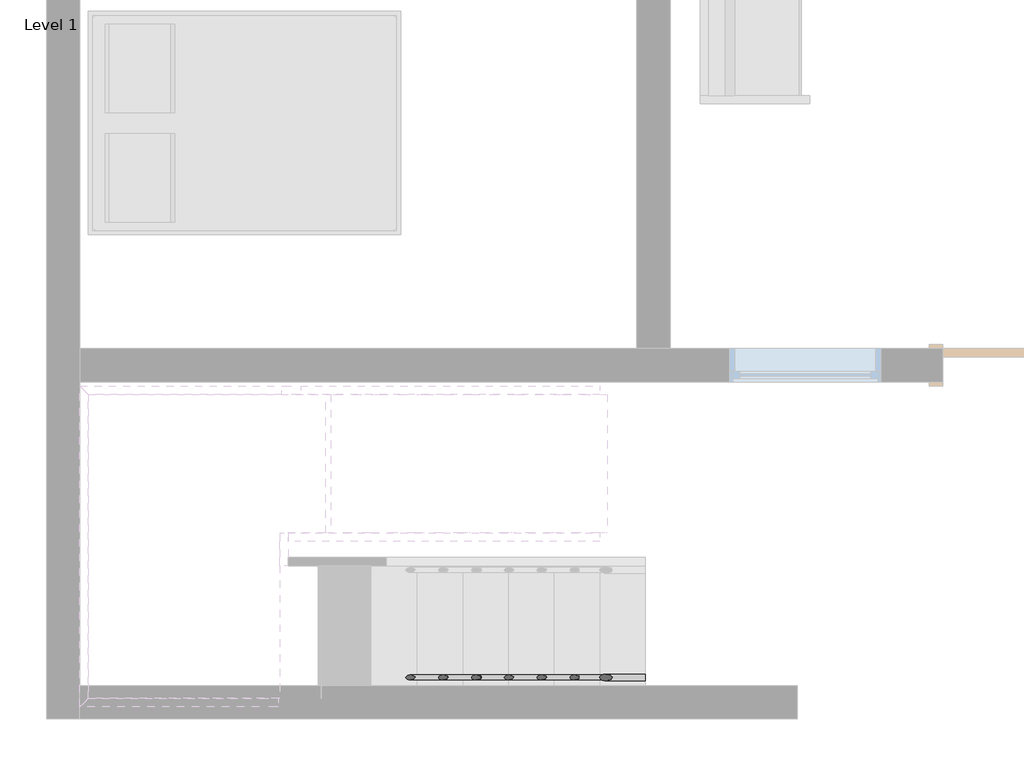
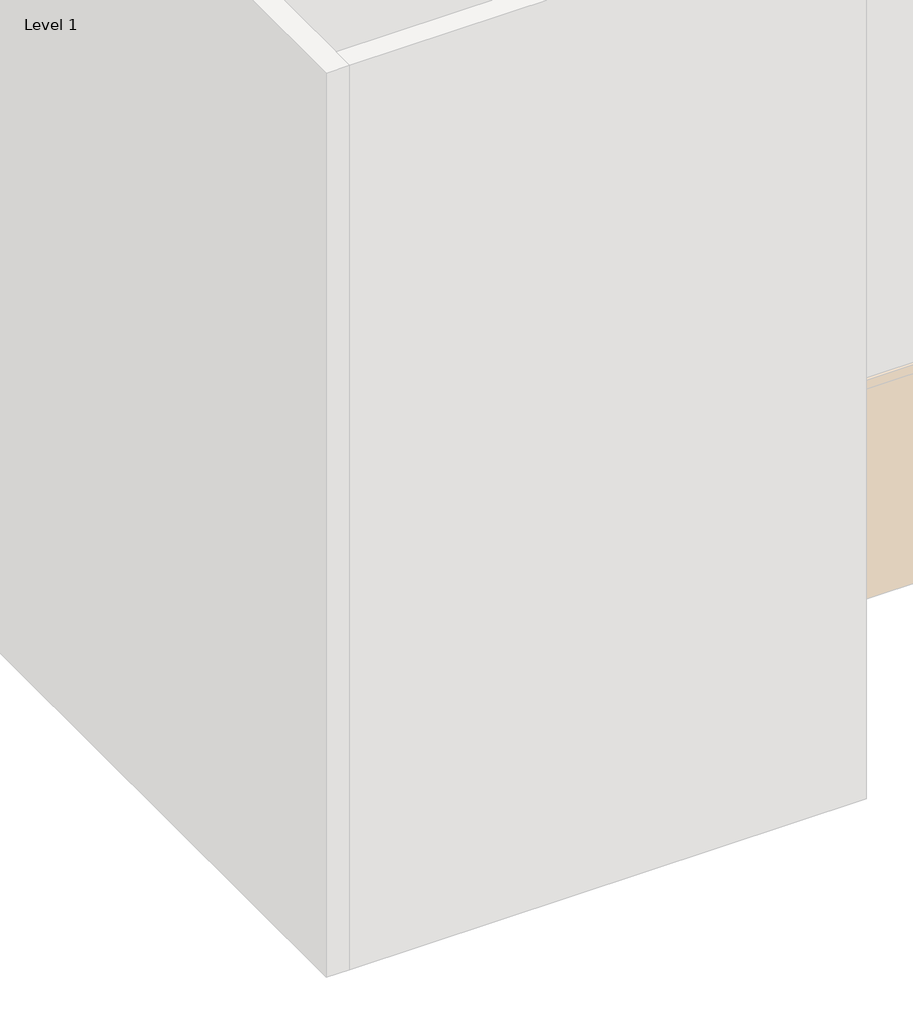
# One storey, part 3 of 4: 1 railing.
"""IFC4 building model written with IfcOpenShell, lengths in millimetres."""

from ifc_helpers import new_model, si_unit, point, frame, frame_2d, origin, place, context, project, spatial, circle_curve, ellipse_curve, trimmed, segment, composite_curve, outline, extrude, element, save
from ifc_brep_helpers import plane_surface, cylinder_surface, advanced_brep

model = new_model("IFC4")

# Units and contexts
model_context = context("Model", 3, world=origin())
ifc_project = project(units=[si_unit("LENGTHUNIT", "METRE", prefix="MILLI")], contexts=[model_context])

# Site, building, storey
site = spatial("IfcSite", under=ifc_project)
building = spatial("IfcBuilding", under=site)
storey = spatial("IfcBuildingStorey", under=building, Name="Level 1", Elevation=0.0)

# Railing
placement = place(None, origin())
element("IfcRailing", 1, ObjectType="900mm Pipe", at=placement, inside=storey, context=model_context, shape_type="SolidModel", body=[
    advanced_brep(
    [(-7153.6870075, 1559.2865734, 1050.2491997), (-7153.6870075, 1519.2865734, 1050.2491997), (-9359.4804605, 1559.2865734, 2445.2173913), (-9359.4804605, 1519.2865734, 2445.2173913), (-10462.6870075, 1559.2865734, 2445.2173913), (-10502.6870075, 1519.2865734, 2445.2173913), (-10462.6870075, 3300.4865734, 2445.2173913), (-10502.6870075, 3340.4865734, 2445.2173913), (-7428.6870075, 3300.4865734, 2445.2173913), (-7428.6870075, 3340.4865734, 2445.2173913)],
    [
        (0, 1, ellipse_curve(frame((-7153.6870075, 1539.2865734, 1050.2491997), z_axis=(1.0, 0.0, 0.0), x_axis=(0.0, 0.0, -1.0)), 23.6638438, 20.0)),
        (1, 0, ellipse_curve(frame((-7153.6870075, 1539.2865734, 1050.2491997), z_axis=(1.0, 0.0, 0.0), x_axis=(0.0, 0.0, -1.0)), 23.6638438, 20.0)),
        (0, 2),
        (2, 3, ellipse_curve(frame((-9359.4804605, 1539.2865734, 2445.2173913), z_axis=(0.9605132043335072, 0.0, -0.27823440531497556), x_axis=(-0.2782344053149751, 0.0, -0.9605132043335075)), 20.822202, 20.0)),
        (3, 1),
        (3, 2, ellipse_curve(frame((-9359.4804605, 1539.2865734, 2445.2173913), z_axis=(0.9605132043335072, 0.0, -0.27823440531497556), x_axis=(-0.2782344053149751, 0.0, -0.9605132043335075)), 20.822202, 20.0)),
        (2, 4),
        (4, 5, ellipse_curve(frame((-10482.6870075, 1539.2865734, 2445.2173913), z_axis=(0.7071067811865449, -0.70710678118655, 0.0), x_axis=(0.7071067811865501, 0.7071067811865448, 0.0)), 28.2842712, 20.0)),
        (5, 3),
        (5, 4, ellipse_curve(frame((-10482.6870075, 1539.2865734, 2445.2173913), z_axis=(0.7071067811865449, -0.70710678118655, 0.0), x_axis=(0.7071067811865501, 0.7071067811865448, 0.0)), 28.2842712, 20.0)),
        (4, 6),
        (6, 7, ellipse_curve(frame((-10482.6870075, 3320.4865734, 2445.2173913), z_axis=(-0.70710678118655, -0.7071067811865451, 0.0), x_axis=(0.7071067811865451, -0.7071067811865498, 0.0)), 28.2842712, 20.0)),
        (7, 5),
        (7, 6, ellipse_curve(frame((-10482.6870075, 3320.4865734, 2445.2173913), z_axis=(-0.70710678118655, -0.7071067811865451, 0.0), x_axis=(0.7071067811865451, -0.7071067811865498, 0.0)), 28.2842712, 20.0)),
        (8, 9, circle_curve(frame((-7428.6870075, 3320.4865734, 2445.2173913), z_axis=(1.0, 0.0, 0.0), x_axis=(0.0, 1.0, 0.0)), 20.0)),
        (9, 8, circle_curve(frame((-7428.6870075, 3320.4865734, 2445.2173913), z_axis=(1.0, 0.0, 0.0), x_axis=(0.0, 1.0, 0.0)), 20.0)),
        (6, 8),
        (9, 7),
    ],
    [
        plane_surface(frame((-7153.6870075, 1539.2865734, 1073.9130435), z_axis=(1.0, 0.0, 0.0), x_axis=(0.0, -1.0, 0.0))),
        cylinder_surface(frame((-7164.3769203, 1539.2865734, 1057.0096189), z_axis=(0.8451712313980437, 0.0, -0.5344956404098302), x_axis=(0.0, -1.0, 0.0)), 20.0),
        cylinder_surface(frame((-9353.6870075, 1539.2865734, 2445.2173913), z_axis=(1.0, 0.0, 0.0), x_axis=(0.0, -1.0, 0.0)), 20.0),
        cylinder_surface(frame((-10482.6870075, 1539.2865734, 2445.2173913), z_axis=(0.0, -1.0, 0.0), x_axis=(-1.0, 0.0, 0.0)), 20.0),
        plane_surface(frame((-7428.6870075, 3320.4865734, 2465.2173913), z_axis=(1.0, 0.0, 0.0), x_axis=(0.0, 1.0, 0.0))),
        cylinder_surface(frame((-10482.6870075, 3320.4865734, 2445.2173913), z_axis=(-1.0, 0.0, 0.0), x_axis=(0.0, 1.0, 0.0)), 20.0),
    ],
    [
        (0, [[1, 2]]),
        (1, [[-1, 3, 4, 5]]),
        (1, [[-2, -5, 6, -3]]),
        (2, [[-4, 7, 8, 9]]),
        (2, [[-6, -9, 10, -7]]),
        (3, [[-8, 11, 12, 13]]),
        (3, [[-10, -13, 14, -11]]),
        (4, [[15, 16]]),
        (5, [[-12, 17, -16, 18]]),
        (5, [[-14, -18, -15, -17]]),
    ],
),
    advanced_brep(
    [(-7153.6870075, 1554.2865734, 931.1651606), (-7153.6870075, 1524.2865734, 931.1651606), (-9358.0320973, 1554.2865734, 2325.2173913), (-9358.0320973, 1524.2865734, 2325.2173913), (-10467.6870075, 1554.2865734, 2325.2173913), (-10497.6870075, 1524.2865734, 2325.2173913), (-10467.6870075, 3305.4865734, 2325.2173913), (-10497.6870075, 3335.4865734, 2325.2173913), (-7428.6870075, 3305.4865734, 2325.2173913), (-7428.6870075, 3335.4865734, 2325.2173913)],
    [
        (0, 1, ellipse_curve(frame((-7153.6870075, 1539.2865734, 931.1651606), z_axis=(1.0, 0.0, 0.0), x_axis=(0.0, 0.0, -1.0)), 17.7478828, 15.0)),
        (1, 0, ellipse_curve(frame((-7153.6870075, 1539.2865734, 931.1651606), z_axis=(1.0, 0.0, 0.0), x_axis=(0.0, 0.0, -1.0)), 17.7478828, 15.0)),
        (0, 2),
        (2, 3, ellipse_curve(frame((-9358.0320973, 1539.2865734, 2325.2173913), z_axis=(0.9605132043335072, 0.0, -0.27823440531497556), x_axis=(-0.2782344053149751, 0.0, -0.9605132043335075)), 15.6166515, 15.0)),
        (3, 1),
        (3, 2, ellipse_curve(frame((-9358.0320973, 1539.2865734, 2325.2173913), z_axis=(0.9605132043335072, 0.0, -0.27823440531497556), x_axis=(-0.2782344053149751, 0.0, -0.9605132043335075)), 15.6166515, 15.0)),
        (2, 4),
        (4, 5, ellipse_curve(frame((-10482.6870075, 1539.2865734, 2325.2173913), z_axis=(0.7071067811865449, -0.70710678118655, 0.0), x_axis=(0.7071067811865501, 0.7071067811865448, 0.0)), 21.2132034, 15.0)),
        (5, 3),
        (5, 4, ellipse_curve(frame((-10482.6870075, 1539.2865734, 2325.2173913), z_axis=(0.7071067811865449, -0.70710678118655, 0.0), x_axis=(0.7071067811865501, 0.7071067811865448, 0.0)), 21.2132034, 15.0)),
        (4, 6),
        (6, 7, ellipse_curve(frame((-10482.6870075, 3320.4865734, 2325.2173913), z_axis=(-0.70710678118655, -0.7071067811865451, 0.0), x_axis=(0.7071067811865451, -0.7071067811865498, 0.0)), 21.2132034, 15.0)),
        (7, 5),
        (7, 6, ellipse_curve(frame((-10482.6870075, 3320.4865734, 2325.2173913), z_axis=(-0.70710678118655, -0.7071067811865451, 0.0), x_axis=(0.7071067811865451, -0.7071067811865498, 0.0)), 21.2132034, 15.0)),
        (8, 9, circle_curve(frame((-7428.6870075, 3320.4865734, 2325.2173913), z_axis=(1.0, 0.0, 0.0), x_axis=(0.0, 1.0, 0.0)), 15.0)),
        (9, 8, circle_curve(frame((-7428.6870075, 3320.4865734, 2325.2173913), z_axis=(1.0, 0.0, 0.0), x_axis=(0.0, 1.0, 0.0)), 15.0)),
        (6, 8),
        (9, 7),
    ],
    [
        plane_surface(frame((-7153.6870075, 1539.2865734, 948.9130435), z_axis=(1.0, 0.0, 0.0), x_axis=(0.0, -1.0, 0.0))),
        cylinder_surface(frame((-7161.7044421, 1539.2865734, 936.235475), z_axis=(0.8451712313980437, 0.0, -0.5344956404098302), x_axis=(0.0, -1.0, 0.0)), 15.0),
        cylinder_surface(frame((-9353.6870075, 1539.2865734, 2325.2173913), z_axis=(1.0, 0.0, 0.0), x_axis=(0.0, -1.0, 0.0)), 15.0),
        cylinder_surface(frame((-10482.6870075, 1539.2865734, 2325.2173913), z_axis=(0.0, -1.0, 0.0), x_axis=(-1.0, 0.0, 0.0)), 15.0),
        plane_surface(frame((-7428.6870075, 3320.4865734, 2340.2173913), z_axis=(1.0, 0.0, 0.0), x_axis=(0.0, 1.0, 0.0))),
        cylinder_surface(frame((-10482.6870075, 3320.4865734, 2325.2173913), z_axis=(-1.0, 0.0, 0.0), x_axis=(0.0, 1.0, 0.0)), 15.0),
    ],
    [
        (0, [[1, 2]]),
        (1, [[-1, 3, 4, 5]]),
        (1, [[-2, -5, 6, -3]]),
        (2, [[-4, 7, 8, 9]]),
        (2, [[-6, -9, 10, -7]]),
        (3, [[-8, 11, 12, 13]]),
        (3, [[-10, -13, 14, -11]]),
        (4, [[15, 16]]),
        (5, [[-12, 17, -16, 18]]),
        (5, [[-14, -18, -15, -17]]),
    ],
),
    advanced_brep(
    [(-7153.6870075, 1554.2865734, 806.1651606), (-7153.6870075, 1524.2865734, 806.1651606), (-9358.0320973, 1554.2865734, 2200.2173913), (-9358.0320973, 1524.2865734, 2200.2173913), (-10467.6870075, 1554.2865734, 2200.2173913), (-10497.6870075, 1524.2865734, 2200.2173913), (-10467.6870075, 3305.4865734, 2200.2173913), (-10497.6870075, 3335.4865734, 2200.2173913), (-7428.6870075, 3305.4865734, 2200.2173913), (-7428.6870075, 3335.4865734, 2200.2173913)],
    [
        (0, 1, ellipse_curve(frame((-7153.6870075, 1539.2865734, 806.1651606), z_axis=(1.0, 0.0, 0.0), x_axis=(0.0, 0.0, -1.0)), 17.7478828, 15.0)),
        (1, 0, ellipse_curve(frame((-7153.6870075, 1539.2865734, 806.1651606), z_axis=(1.0, 0.0, 0.0), x_axis=(0.0, 0.0, -1.0)), 17.7478828, 15.0)),
        (0, 2),
        (2, 3, ellipse_curve(frame((-9358.0320973, 1539.2865734, 2200.2173913), z_axis=(0.9605132043335072, 0.0, -0.27823440531497556), x_axis=(-0.2782344053149751, 0.0, -0.9605132043335075)), 15.6166515, 15.0)),
        (3, 1),
        (3, 2, ellipse_curve(frame((-9358.0320973, 1539.2865734, 2200.2173913), z_axis=(0.9605132043335072, 0.0, -0.27823440531497556), x_axis=(-0.2782344053149751, 0.0, -0.9605132043335075)), 15.6166515, 15.0)),
        (2, 4),
        (4, 5, ellipse_curve(frame((-10482.6870075, 1539.2865734, 2200.2173913), z_axis=(0.7071067811865449, -0.70710678118655, 0.0), x_axis=(0.7071067811865501, 0.7071067811865448, 0.0)), 21.2132034, 15.0)),
        (5, 3),
        (5, 4, ellipse_curve(frame((-10482.6870075, 1539.2865734, 2200.2173913), z_axis=(0.7071067811865449, -0.70710678118655, 0.0), x_axis=(0.7071067811865501, 0.7071067811865448, 0.0)), 21.2132034, 15.0)),
        (4, 6),
        (6, 7, ellipse_curve(frame((-10482.6870075, 3320.4865734, 2200.2173913), z_axis=(-0.70710678118655, -0.7071067811865451, 0.0), x_axis=(0.7071067811865451, -0.7071067811865498, 0.0)), 21.2132034, 15.0)),
        (7, 5),
        (7, 6, ellipse_curve(frame((-10482.6870075, 3320.4865734, 2200.2173913), z_axis=(-0.70710678118655, -0.7071067811865451, 0.0), x_axis=(0.7071067811865451, -0.7071067811865498, 0.0)), 21.2132034, 15.0)),
        (8, 9, circle_curve(frame((-7428.6870075, 3320.4865734, 2200.2173913), z_axis=(1.0, 0.0, 0.0), x_axis=(0.0, 1.0, 0.0)), 15.0)),
        (9, 8, circle_curve(frame((-7428.6870075, 3320.4865734, 2200.2173913), z_axis=(1.0, 0.0, 0.0), x_axis=(0.0, 1.0, 0.0)), 15.0)),
        (6, 8),
        (9, 7),
    ],
    [
        plane_surface(frame((-7153.6870075, 1539.2865734, 823.9130435), z_axis=(1.0, 0.0, 0.0), x_axis=(0.0, -1.0, 0.0))),
        cylinder_surface(frame((-7161.7044421, 1539.2865734, 811.235475), z_axis=(0.8451712313980437, 0.0, -0.5344956404098302), x_axis=(0.0, -1.0, 0.0)), 15.0),
        cylinder_surface(frame((-9353.6870075, 1539.2865734, 2200.2173913), z_axis=(1.0, 0.0, 0.0), x_axis=(0.0, -1.0, 0.0)), 15.0),
        cylinder_surface(frame((-10482.6870075, 1539.2865734, 2200.2173913), z_axis=(0.0, -1.0, 0.0), x_axis=(-1.0, 0.0, 0.0)), 15.0),
        plane_surface(frame((-7428.6870075, 3320.4865734, 2215.2173913), z_axis=(1.0, 0.0, 0.0), x_axis=(0.0, 1.0, 0.0))),
        cylinder_surface(frame((-10482.6870075, 3320.4865734, 2200.2173913), z_axis=(-1.0, 0.0, 0.0), x_axis=(0.0, 1.0, 0.0)), 15.0),
    ],
    [
        (0, [[1, 2]]),
        (1, [[-1, 3, 4, 5]]),
        (1, [[-2, -5, 6, -3]]),
        (2, [[-4, 7, 8, 9]]),
        (2, [[-6, -9, 10, -7]]),
        (3, [[-8, 11, 12, 13]]),
        (3, [[-10, -13, 14, -11]]),
        (4, [[15, 16]]),
        (5, [[-12, 17, -16, 18]]),
        (5, [[-14, -18, -15, -17]]),
    ],
),
    advanced_brep(
    [(-7153.6870075, 1554.2865734, 681.1651606), (-7153.6870075, 1524.2865734, 681.1651606), (-9358.0320973, 1554.2865734, 2075.2173913), (-9358.0320973, 1524.2865734, 2075.2173913), (-10467.6870075, 1554.2865734, 2075.2173913), (-10497.6870075, 1524.2865734, 2075.2173913), (-10467.6870075, 3305.4865734, 2075.2173913), (-10497.6870075, 3335.4865734, 2075.2173913), (-7428.6870075, 3305.4865734, 2075.2173913), (-7428.6870075, 3335.4865734, 2075.2173913)],
    [
        (0, 1, ellipse_curve(frame((-7153.6870075, 1539.2865734, 681.1651606), z_axis=(1.0, 0.0, 0.0), x_axis=(0.0, 0.0, -1.0)), 17.7478828, 15.0)),
        (1, 0, ellipse_curve(frame((-7153.6870075, 1539.2865734, 681.1651606), z_axis=(1.0, 0.0, 0.0), x_axis=(0.0, 0.0, -1.0)), 17.7478828, 15.0)),
        (0, 2),
        (2, 3, ellipse_curve(frame((-9358.0320973, 1539.2865734, 2075.2173913), z_axis=(0.9605132043335072, 0.0, -0.27823440531497556), x_axis=(-0.2782344053149751, 0.0, -0.9605132043335075)), 15.6166515, 15.0)),
        (3, 1),
        (3, 2, ellipse_curve(frame((-9358.0320973, 1539.2865734, 2075.2173913), z_axis=(0.9605132043335072, 0.0, -0.27823440531497556), x_axis=(-0.2782344053149751, 0.0, -0.9605132043335075)), 15.6166515, 15.0)),
        (2, 4),
        (4, 5, ellipse_curve(frame((-10482.6870075, 1539.2865734, 2075.2173913), z_axis=(0.7071067811865449, -0.70710678118655, 0.0), x_axis=(0.7071067811865501, 0.7071067811865448, 0.0)), 21.2132034, 15.0)),
        (5, 3),
        (5, 4, ellipse_curve(frame((-10482.6870075, 1539.2865734, 2075.2173913), z_axis=(0.7071067811865449, -0.70710678118655, 0.0), x_axis=(0.7071067811865501, 0.7071067811865448, 0.0)), 21.2132034, 15.0)),
        (4, 6),
        (6, 7, ellipse_curve(frame((-10482.6870075, 3320.4865734, 2075.2173913), z_axis=(-0.70710678118655, -0.7071067811865451, 0.0), x_axis=(0.7071067811865451, -0.7071067811865498, 0.0)), 21.2132034, 15.0)),
        (7, 5),
        (7, 6, ellipse_curve(frame((-10482.6870075, 3320.4865734, 2075.2173913), z_axis=(-0.70710678118655, -0.7071067811865451, 0.0), x_axis=(0.7071067811865451, -0.7071067811865498, 0.0)), 21.2132034, 15.0)),
        (8, 9, circle_curve(frame((-7428.6870075, 3320.4865734, 2075.2173913), z_axis=(1.0, 0.0, 0.0), x_axis=(0.0, 1.0, 0.0)), 15.0)),
        (9, 8, circle_curve(frame((-7428.6870075, 3320.4865734, 2075.2173913), z_axis=(1.0, 0.0, 0.0), x_axis=(0.0, 1.0, 0.0)), 15.0)),
        (6, 8),
        (9, 7),
    ],
    [
        plane_surface(frame((-7153.6870075, 1539.2865734, 698.9130435), z_axis=(1.0, 0.0, 0.0), x_axis=(0.0, -1.0, 0.0))),
        cylinder_surface(frame((-7161.7044421, 1539.2865734, 686.235475), z_axis=(0.8451712313980437, 0.0, -0.5344956404098302), x_axis=(0.0, -1.0, 0.0)), 15.0),
        cylinder_surface(frame((-9353.6870075, 1539.2865734, 2075.2173913), z_axis=(1.0, 0.0, 0.0), x_axis=(0.0, -1.0, 0.0)), 15.0),
        cylinder_surface(frame((-10482.6870075, 1539.2865734, 2075.2173913), z_axis=(0.0, -1.0, 0.0), x_axis=(-1.0, 0.0, 0.0)), 15.0),
        plane_surface(frame((-7428.6870075, 3320.4865734, 2090.2173913), z_axis=(1.0, 0.0, 0.0), x_axis=(0.0, 1.0, 0.0))),
        cylinder_surface(frame((-10482.6870075, 3320.4865734, 2075.2173913), z_axis=(-1.0, 0.0, 0.0), x_axis=(0.0, 1.0, 0.0)), 15.0),
    ],
    [
        (0, [[1, 2]]),
        (1, [[-1, 3, 4, 5]]),
        (1, [[-2, -5, 6, -3]]),
        (2, [[-4, 7, 8, 9]]),
        (2, [[-6, -9, 10, -7]]),
        (3, [[-8, 11, 12, 13]]),
        (3, [[-10, -13, 14, -11]]),
        (4, [[15, 16]]),
        (5, [[-12, 17, -16, 18]]),
        (5, [[-14, -18, -15, -17]]),
    ],
),
    advanced_brep(
    [(-7153.6870075, 1554.2865734, 556.1651606), (-7153.6870075, 1524.2865734, 556.1651606), (-9358.0320973, 1554.2865734, 1950.2173913), (-9358.0320973, 1524.2865734, 1950.2173913), (-10467.6870075, 1554.2865734, 1950.2173913), (-10497.6870075, 1524.2865734, 1950.2173913), (-10467.6870075, 3305.4865734, 1950.2173913), (-10497.6870075, 3335.4865734, 1950.2173913), (-7428.6870075, 3305.4865734, 1950.2173913), (-7428.6870075, 3335.4865734, 1950.2173913)],
    [
        (0, 1, ellipse_curve(frame((-7153.6870075, 1539.2865734, 556.1651606), z_axis=(1.0, 0.0, 0.0), x_axis=(0.0, 0.0, -1.0)), 17.7478828, 15.0)),
        (1, 0, ellipse_curve(frame((-7153.6870075, 1539.2865734, 556.1651606), z_axis=(1.0, 0.0, 0.0), x_axis=(0.0, 0.0, -1.0)), 17.7478828, 15.0)),
        (0, 2),
        (2, 3, ellipse_curve(frame((-9358.0320973, 1539.2865734, 1950.2173913), z_axis=(0.9605132043335072, 0.0, -0.27823440531497556), x_axis=(-0.2782344053149751, 0.0, -0.9605132043335075)), 15.6166515, 15.0)),
        (3, 1),
        (3, 2, ellipse_curve(frame((-9358.0320973, 1539.2865734, 1950.2173913), z_axis=(0.9605132043335072, 0.0, -0.27823440531497556), x_axis=(-0.2782344053149751, 0.0, -0.9605132043335075)), 15.6166515, 15.0)),
        (2, 4),
        (4, 5, ellipse_curve(frame((-10482.6870075, 1539.2865734, 1950.2173913), z_axis=(0.7071067811865449, -0.70710678118655, 0.0), x_axis=(0.7071067811865501, 0.7071067811865448, 0.0)), 21.2132034, 15.0)),
        (5, 3),
        (5, 4, ellipse_curve(frame((-10482.6870075, 1539.2865734, 1950.2173913), z_axis=(0.7071067811865449, -0.70710678118655, 0.0), x_axis=(0.7071067811865501, 0.7071067811865448, 0.0)), 21.2132034, 15.0)),
        (4, 6),
        (6, 7, ellipse_curve(frame((-10482.6870075, 3320.4865734, 1950.2173913), z_axis=(-0.70710678118655, -0.7071067811865451, 0.0), x_axis=(0.7071067811865451, -0.7071067811865498, 0.0)), 21.2132034, 15.0)),
        (7, 5),
        (7, 6, ellipse_curve(frame((-10482.6870075, 3320.4865734, 1950.2173913), z_axis=(-0.70710678118655, -0.7071067811865451, 0.0), x_axis=(0.7071067811865451, -0.7071067811865498, 0.0)), 21.2132034, 15.0)),
        (8, 9, circle_curve(frame((-7428.6870075, 3320.4865734, 1950.2173913), z_axis=(1.0, 0.0, 0.0), x_axis=(0.0, 1.0, 0.0)), 15.0)),
        (9, 8, circle_curve(frame((-7428.6870075, 3320.4865734, 1950.2173913), z_axis=(1.0, 0.0, 0.0), x_axis=(0.0, 1.0, 0.0)), 15.0)),
        (6, 8),
        (9, 7),
    ],
    [
        plane_surface(frame((-7153.6870075, 1539.2865734, 573.9130435), z_axis=(1.0, 0.0, 0.0), x_axis=(0.0, -1.0, 0.0))),
        cylinder_surface(frame((-7161.7044421, 1539.2865734, 561.235475), z_axis=(0.8451712313980437, 0.0, -0.5344956404098302), x_axis=(0.0, -1.0, 0.0)), 15.0),
        cylinder_surface(frame((-9353.6870075, 1539.2865734, 1950.2173913), z_axis=(1.0, 0.0, 0.0), x_axis=(0.0, -1.0, 0.0)), 15.0),
        cylinder_surface(frame((-10482.6870075, 1539.2865734, 1950.2173913), z_axis=(0.0, -1.0, 0.0), x_axis=(-1.0, 0.0, 0.0)), 15.0),
        plane_surface(frame((-7428.6870075, 3320.4865734, 1965.2173913), z_axis=(1.0, 0.0, 0.0), x_axis=(0.0, 1.0, 0.0))),
        cylinder_surface(frame((-10482.6870075, 3320.4865734, 1950.2173913), z_axis=(-1.0, 0.0, 0.0), x_axis=(0.0, 1.0, 0.0)), 15.0),
    ],
    [
        (0, [[1, 2]]),
        (1, [[-1, 3, 4, 5]]),
        (1, [[-2, -5, 6, -3]]),
        (2, [[-4, 7, 8, 9]]),
        (2, [[-6, -9, 10, -7]]),
        (3, [[-8, 11, 12, 13]]),
        (3, [[-10, -13, 14, -11]]),
        (4, [[15, 16]]),
        (5, [[-12, 17, -16, 18]]),
        (5, [[-14, -18, -15, -17]]),
    ],
),
    advanced_brep(
    [(-7153.6870075, 1554.2865734, 431.1651606), (-7153.6870075, 1524.2865734, 431.1651606), (-9358.0320973, 1554.2865734, 1825.2173913), (-9358.0320973, 1524.2865734, 1825.2173913), (-10467.6870075, 1554.2865734, 1825.2173913), (-10497.6870075, 1524.2865734, 1825.2173913), (-10467.6870075, 3305.4865734, 1825.2173913), (-10497.6870075, 3335.4865734, 1825.2173913), (-7428.6870075, 3305.4865734, 1825.2173913), (-7428.6870075, 3335.4865734, 1825.2173913)],
    [
        (0, 1, ellipse_curve(frame((-7153.6870075, 1539.2865734, 431.1651606), z_axis=(1.0, 0.0, 0.0), x_axis=(0.0, 0.0, -1.0)), 17.7478828, 15.0)),
        (1, 0, ellipse_curve(frame((-7153.6870075, 1539.2865734, 431.1651606), z_axis=(1.0, 0.0, 0.0), x_axis=(0.0, 0.0, -1.0)), 17.7478828, 15.0)),
        (0, 2),
        (2, 3, ellipse_curve(frame((-9358.0320973, 1539.2865734, 1825.2173913), z_axis=(0.9605132043335072, 0.0, -0.27823440531497556), x_axis=(-0.2782344053149751, 0.0, -0.9605132043335075)), 15.6166515, 15.0)),
        (3, 1),
        (3, 2, ellipse_curve(frame((-9358.0320973, 1539.2865734, 1825.2173913), z_axis=(0.9605132043335072, 0.0, -0.27823440531497556), x_axis=(-0.2782344053149751, 0.0, -0.9605132043335075)), 15.6166515, 15.0)),
        (2, 4),
        (4, 5, ellipse_curve(frame((-10482.6870075, 1539.2865734, 1825.2173913), z_axis=(0.7071067811865449, -0.70710678118655, 0.0), x_axis=(0.7071067811865501, 0.7071067811865448, 0.0)), 21.2132034, 15.0)),
        (5, 3),
        (5, 4, ellipse_curve(frame((-10482.6870075, 1539.2865734, 1825.2173913), z_axis=(0.7071067811865449, -0.70710678118655, 0.0), x_axis=(0.7071067811865501, 0.7071067811865448, 0.0)), 21.2132034, 15.0)),
        (4, 6),
        (6, 7, ellipse_curve(frame((-10482.6870075, 3320.4865734, 1825.2173913), z_axis=(-0.70710678118655, -0.7071067811865451, 0.0), x_axis=(0.7071067811865451, -0.7071067811865498, 0.0)), 21.2132034, 15.0)),
        (7, 5),
        (7, 6, ellipse_curve(frame((-10482.6870075, 3320.4865734, 1825.2173913), z_axis=(-0.70710678118655, -0.7071067811865451, 0.0), x_axis=(0.7071067811865451, -0.7071067811865498, 0.0)), 21.2132034, 15.0)),
        (8, 9, circle_curve(frame((-7428.6870075, 3320.4865734, 1825.2173913), z_axis=(1.0, 0.0, 0.0), x_axis=(0.0, 1.0, 0.0)), 15.0)),
        (9, 8, circle_curve(frame((-7428.6870075, 3320.4865734, 1825.2173913), z_axis=(1.0, 0.0, 0.0), x_axis=(0.0, 1.0, 0.0)), 15.0)),
        (6, 8),
        (9, 7),
    ],
    [
        plane_surface(frame((-7153.6870075, 1539.2865734, 448.9130435), z_axis=(1.0, 0.0, 0.0), x_axis=(0.0, -1.0, 0.0))),
        cylinder_surface(frame((-7161.7044421, 1539.2865734, 436.235475), z_axis=(0.8451712313980437, 0.0, -0.5344956404098302), x_axis=(0.0, -1.0, 0.0)), 15.0),
        cylinder_surface(frame((-9353.6870075, 1539.2865734, 1825.2173913), z_axis=(1.0, 0.0, 0.0), x_axis=(0.0, -1.0, 0.0)), 15.0),
        cylinder_surface(frame((-10482.6870075, 1539.2865734, 1825.2173913), z_axis=(0.0, -1.0, 0.0), x_axis=(-1.0, 0.0, 0.0)), 15.0),
        plane_surface(frame((-7428.6870075, 3320.4865734, 1840.2173913), z_axis=(1.0, 0.0, 0.0), x_axis=(0.0, 1.0, 0.0))),
        cylinder_surface(frame((-10482.6870075, 3320.4865734, 1825.2173913), z_axis=(-1.0, 0.0, 0.0), x_axis=(0.0, 1.0, 0.0)), 15.0),
    ],
    [
        (0, [[1, 2]]),
        (1, [[-1, 3, 4, 5]]),
        (1, [[-2, -5, 6, -3]]),
        (2, [[-4, 7, 8, 9]]),
        (2, [[-6, -9, 10, -7]]),
        (3, [[-8, 11, 12, 13]]),
        (3, [[-10, -13, 14, -11]]),
        (4, [[15, 16]]),
        (5, [[-12, 17, -16, 18]]),
        (5, [[-14, -18, -15, -17]]),
    ],
),
    advanced_brep(
    [(-7153.6870075, 1554.2865734, 306.1651606), (-7153.6870075, 1524.2865734, 306.1651606), (-9358.0320973, 1554.2865734, 1700.2173913), (-9358.0320973, 1524.2865734, 1700.2173913), (-10467.6870075, 1554.2865734, 1700.2173913), (-10497.6870075, 1524.2865734, 1700.2173913), (-10467.6870075, 3305.4865734, 1700.2173913), (-10497.6870075, 3335.4865734, 1700.2173913), (-7428.6870075, 3305.4865734, 1700.2173913), (-7428.6870075, 3335.4865734, 1700.2173913)],
    [
        (0, 1, ellipse_curve(frame((-7153.6870075, 1539.2865734, 306.1651606), z_axis=(1.0, 0.0, 0.0), x_axis=(0.0, 0.0, -1.0)), 17.7478828, 15.0)),
        (1, 0, ellipse_curve(frame((-7153.6870075, 1539.2865734, 306.1651606), z_axis=(1.0, 0.0, 0.0), x_axis=(0.0, 0.0, -1.0)), 17.7478828, 15.0)),
        (0, 2),
        (2, 3, ellipse_curve(frame((-9358.0320973, 1539.2865734, 1700.2173913), z_axis=(0.9605132043335072, 0.0, -0.27823440531497556), x_axis=(-0.2782344053149751, 0.0, -0.9605132043335075)), 15.6166515, 15.0)),
        (3, 1),
        (3, 2, ellipse_curve(frame((-9358.0320973, 1539.2865734, 1700.2173913), z_axis=(0.9605132043335072, 0.0, -0.27823440531497556), x_axis=(-0.2782344053149751, 0.0, -0.9605132043335075)), 15.6166515, 15.0)),
        (2, 4),
        (4, 5, ellipse_curve(frame((-10482.6870075, 1539.2865734, 1700.2173913), z_axis=(0.7071067811865449, -0.70710678118655, 0.0), x_axis=(0.7071067811865501, 0.7071067811865448, 0.0)), 21.2132034, 15.0)),
        (5, 3),
        (5, 4, ellipse_curve(frame((-10482.6870075, 1539.2865734, 1700.2173913), z_axis=(0.7071067811865449, -0.70710678118655, 0.0), x_axis=(0.7071067811865501, 0.7071067811865448, 0.0)), 21.2132034, 15.0)),
        (4, 6),
        (6, 7, ellipse_curve(frame((-10482.6870075, 3320.4865734, 1700.2173913), z_axis=(-0.70710678118655, -0.7071067811865451, 0.0), x_axis=(0.7071067811865451, -0.7071067811865498, 0.0)), 21.2132034, 15.0)),
        (7, 5),
        (7, 6, ellipse_curve(frame((-10482.6870075, 3320.4865734, 1700.2173913), z_axis=(-0.70710678118655, -0.7071067811865451, 0.0), x_axis=(0.7071067811865451, -0.7071067811865498, 0.0)), 21.2132034, 15.0)),
        (8, 9, circle_curve(frame((-7428.6870075, 3320.4865734, 1700.2173913), z_axis=(1.0, 0.0, 0.0), x_axis=(0.0, 1.0, 0.0)), 15.0)),
        (9, 8, circle_curve(frame((-7428.6870075, 3320.4865734, 1700.2173913), z_axis=(1.0, 0.0, 0.0), x_axis=(0.0, 1.0, 0.0)), 15.0)),
        (6, 8),
        (9, 7),
    ],
    [
        plane_surface(frame((-7153.6870075, 1539.2865734, 323.9130435), z_axis=(1.0, 0.0, 0.0), x_axis=(0.0, -1.0, 0.0))),
        cylinder_surface(frame((-7161.7044421, 1539.2865734, 311.235475), z_axis=(0.8451712313980437, 0.0, -0.5344956404098302), x_axis=(0.0, -1.0, 0.0)), 15.0),
        cylinder_surface(frame((-9353.6870075, 1539.2865734, 1700.2173913), z_axis=(1.0, 0.0, 0.0), x_axis=(0.0, -1.0, 0.0)), 15.0),
        cylinder_surface(frame((-10482.6870075, 1539.2865734, 1700.2173913), z_axis=(0.0, -1.0, 0.0), x_axis=(-1.0, 0.0, 0.0)), 15.0),
        plane_surface(frame((-7428.6870075, 3320.4865734, 1715.2173913), z_axis=(1.0, 0.0, 0.0), x_axis=(0.0, 1.0, 0.0))),
        cylinder_surface(frame((-10482.6870075, 3320.4865734, 1700.2173913), z_axis=(-1.0, 0.0, 0.0), x_axis=(0.0, 1.0, 0.0)), 15.0),
    ],
    [
        (0, [[1, 2]]),
        (1, [[-1, 3, 4, 5]]),
        (1, [[-2, -5, 6, -3]]),
        (2, [[-4, 7, 8, 9]]),
        (2, [[-6, -9, 10, -7]]),
        (3, [[-8, 11, 12, 13]]),
        (3, [[-10, -13, 14, -11]]),
        (4, [[15, 16]]),
        (5, [[-12, 17, -16, 18]]),
        (5, [[-14, -18, -15, -17]]),
    ],
),
    extrude(outline(composite_curve([segment(trimmed(circle_curve(frame_2d((-8078.6870075, 3320.4865734)), 12.5), [point((-8078.6870075, 3307.9865734))], [point((-8078.6870075, 3332.9865734))], False, "CARTESIAN"), True, "CONTINUOUS"), segment(trimmed(circle_curve(frame_2d((-8078.6870075, 3320.4865734)), 12.5), [point((-8078.6870075, 3332.9865734))], [point((-8078.6870075, 3307.9865734))], False, "CARTESIAN"), True, "CONTINUOUS")], self_intersect=False)), frame((0.0, 0.0, 1565.2173913), z_axis=(0.0, 0.0, 1.0), x_axis=(1.0, 0.0, 0.0)), (0.0, 0.0, 1.0), 860.0),
    extrude(outline(composite_curve([segment(trimmed(circle_curve(frame_2d((-9482.6870075, 3320.4865734)), 12.5), [point((-9482.6870075, 3307.9865734))], [point((-9482.6870075, 3332.9865734))], False, "CARTESIAN"), True, "CONTINUOUS"), segment(trimmed(circle_curve(frame_2d((-9482.6870075, 3320.4865734)), 12.5), [point((-9482.6870075, 3332.9865734))], [point((-9482.6870075, 3307.9865734))], False, "CARTESIAN"), True, "CONTINUOUS")], self_intersect=False)), frame((0.0, 0.0, 1565.2173913), z_axis=(0.0, 0.0, 1.0), x_axis=(1.0, 0.0, 0.0)), (0.0, 0.0, 1.0), 860.0),
    extrude(outline(composite_curve([segment(trimmed(circle_curve(frame_2d((-10482.6870075, 2539.2865734)), 12.5), [point((-10470.1870075, 2539.2865734))], [point((-10495.1870075, 2539.2865734))], False, "CARTESIAN"), True, "CONTINUOUS"), segment(trimmed(circle_curve(frame_2d((-10482.6870075, 2539.2865734)), 12.5), [point((-10495.1870075, 2539.2865734))], [point((-10470.1870075, 2539.2865734))], False, "CARTESIAN"), True, "CONTINUOUS")], self_intersect=False)), frame((0.0, 0.0, 1565.2173913), z_axis=(0.0, 0.0, 1.0), x_axis=(1.0, 0.0, 0.0)), (0.0, 0.0, 1.0), 860.0),
    extrude(outline(composite_curve([segment(trimmed(circle_curve(frame_2d((-10353.6870075, 1539.2865734)), 12.5), [point((-10353.6870075, 1551.7865734))], [point((-10353.6870075, 1526.7865734))], False, "CARTESIAN"), True, "CONTINUOUS"), segment(trimmed(circle_curve(frame_2d((-10353.6870075, 1539.2865734)), 12.5), [point((-10353.6870075, 1526.7865734))], [point((-10353.6870075, 1551.7865734))], False, "CARTESIAN"), True, "CONTINUOUS")], self_intersect=False)), frame((0.0, 0.0, 1565.2173913), z_axis=(0.0, 0.0, 1.0), x_axis=(1.0, 0.0, 0.0)), (0.0, 0.0, 1.0), 860.0),
    advanced_brep(
    [(-9153.6870075, 1526.7865734, 2291.4074903), (-9153.6870075, 1551.7865734, 2291.4074903), (-9153.6870075, 1551.7865734, 1391.3043478), (-9153.6870075, 1526.7865734, 1391.3043478)],
    [
        (0, 1, ellipse_curve(frame((-9153.6870075, 1539.2865734, 2291.4074903), z_axis=(-0.5344956404098302, 0.0, -0.8451712313980437), x_axis=(-0.8451712313980437, 0.0, 0.53449564040983)), 14.7899024, 12.5)),
        (1, 2),
        (2, 3, circle_curve(frame((-9153.6870075, 1539.2865734, 1391.3043478), z_axis=(0.0, 0.0, 1.0), x_axis=(0.0, 1.0, 0.0)), 12.5)),
        (3, 0),
        (3, 2, circle_curve(frame((-9153.6870075, 1539.2865734, 1391.3043478), z_axis=(0.0, 0.0, 1.0), x_axis=(0.0, 1.0, 0.0)), 12.5)),
        (1, 0, ellipse_curve(frame((-9153.6870075, 1539.2865734, 2291.4074903), z_axis=(-0.5344956404098302, 0.0, -0.8451712313980437), x_axis=(-0.8451712313980437, 0.0, 0.53449564040983)), 14.7899024, 12.5)),
    ],
    [
        cylinder_surface(frame((-9153.6870075, 1539.2865734, 1291.3043478), z_axis=(0.0, 0.0, 1.0), x_axis=(0.0, 1.0, 0.0)), 12.5),
        plane_surface(frame((-9178.6870075, 1564.2865734, 2307.217767), z_axis=(0.5344956404098302, 0.0, 0.8451712313980437), x_axis=(0.0, -1.0, 0.0))),
        plane_surface(frame((-9128.6870075, 1564.2865734, 1391.3043478), z_axis=(0.0, 0.0, -1.0), x_axis=(0.0, -1.0, 0.0))),
    ],
    [
        (0, [[1, 2, 3, 4]]),
        (0, [[5, -2, 6, -4]]),
        (1, [[-6, -1]]),
        (2, [[-5, -3]]),
    ],
),
    advanced_brep(
    [(-8153.6870075, 1526.7865734, 1658.9964231), (-8153.6870075, 1551.7865734, 1658.9964231), (-8153.6870075, 1551.7865734, 695.6521739), (-8153.6870075, 1526.7865734, 695.6521739)],
    [
        (0, 1, ellipse_curve(frame((-8153.6870075, 1539.2865734, 1658.9964231), z_axis=(-0.5344956404098302, 0.0, -0.8451712313980437), x_axis=(-0.8451712313980437, 0.0, 0.53449564040983)), 14.7899024, 12.5)),
        (1, 2),
        (2, 3, circle_curve(frame((-8153.6870075, 1539.2865734, 695.6521739), z_axis=(0.0, 0.0, 1.0), x_axis=(0.0, 1.0, 0.0)), 12.5)),
        (3, 0),
        (3, 2, circle_curve(frame((-8153.6870075, 1539.2865734, 695.6521739), z_axis=(0.0, 0.0, 1.0), x_axis=(0.0, 1.0, 0.0)), 12.5)),
        (1, 0, ellipse_curve(frame((-8153.6870075, 1539.2865734, 1658.9964231), z_axis=(-0.5344956404098302, 0.0, -0.8451712313980437), x_axis=(-0.8451712313980437, 0.0, 0.53449564040983)), 14.7899024, 12.5)),
    ],
    [
        cylinder_surface(frame((-8153.6870075, 1539.2865734, 595.6521739), z_axis=(0.0, 0.0, 1.0), x_axis=(0.0, 1.0, 0.0)), 12.5),
        plane_surface(frame((-8178.6870075, 1564.2865734, 1674.8066998), z_axis=(0.5344956404098302, 0.0, 0.8451712313980437), x_axis=(0.0, -1.0, 0.0))),
        plane_surface(frame((-8128.6870075, 1564.2865734, 695.6521739), z_axis=(0.0, 0.0, -1.0), x_axis=(0.0, -1.0, 0.0))),
    ],
    [
        (0, [[1, 2, 3, 4]]),
        (0, [[5, -2, 6, -4]]),
        (1, [[-6, -1]]),
        (2, [[-5, -3]]),
    ],
),
    extrude(outline(composite_curve([segment(trimmed(circle_curve(frame_2d((-9078.6870075, 3320.4865734)), 12.5), [point((-9078.6870075, 3307.9865734))], [point((-9078.6870075, 3332.9865734))], False, "CARTESIAN"), True, "CONTINUOUS"), segment(trimmed(circle_curve(frame_2d((-9078.6870075, 3320.4865734)), 12.5), [point((-9078.6870075, 3332.9865734))], [point((-9078.6870075, 3307.9865734))], False, "CARTESIAN"), True, "CONTINUOUS")], self_intersect=False)), frame((0.0, 0.0, 1565.2173913), z_axis=(0.0, 0.0, 1.0), x_axis=(1.0, 0.0, 0.0)), (0.0, 0.0, 1.0), 860.0),
    extrude(outline(composite_curve([segment(trimmed(circle_curve(frame_2d((-10482.6870075, 3320.4865734)), 12.5), [point((-10470.1870075, 3320.4865734))], [point((-10495.1870075, 3320.4865734))], False, "CARTESIAN"), True, "CONTINUOUS"), segment(trimmed(circle_curve(frame_2d((-10482.6870075, 3320.4865734)), 12.5), [point((-10495.1870075, 3320.4865734))], [point((-10470.1870075, 3320.4865734))], False, "CARTESIAN"), True, "CONTINUOUS")], self_intersect=False)), frame((0.0, 0.0, 1565.2173913), z_axis=(0.0, 0.0, 1.0), x_axis=(1.0, 0.0, 0.0)), (0.0, 0.0, 1.0), 860.0),
    extrude(outline(composite_curve([segment(trimmed(circle_curve(frame_2d((-10482.6870075, 1539.2865734)), 12.5), [point((-10482.6870075, 1551.7865734))], [point((-10482.6870075, 1526.7865734))], False, "CARTESIAN"), True, "CONTINUOUS"), segment(trimmed(circle_curve(frame_2d((-10482.6870075, 1539.2865734)), 12.5), [point((-10482.6870075, 1526.7865734))], [point((-10482.6870075, 1551.7865734))], False, "CARTESIAN"), True, "CONTINUOUS")], self_intersect=False)), frame((0.0, 0.0, 1565.2173913), z_axis=(0.0, 0.0, 1.0), x_axis=(1.0, 0.0, 0.0)), (0.0, 0.0, 1.0), 860.0),
    advanced_brep(
    [(-9353.6870075, 1526.7865734, 2417.8897037), (-9353.6870075, 1551.7865734, 2417.8897037), (-9353.6870075, 1551.7865734, 1565.2173913), (-9353.6870075, 1526.7865734, 1565.2173913)],
    [
        (0, 1, ellipse_curve(frame((-9353.6870075, 1539.2865734, 2417.8897037), z_axis=(-0.5344956404098286, 0.0, -0.8451712313980447), x_axis=(-0.8451712313980447, 0.0, 0.5344956404098286)), 14.7899024, 12.5)),
        (1, 2),
        (2, 3, circle_curve(frame((-9353.6870075, 1539.2865734, 1565.2173913), z_axis=(0.0, 0.0, 1.0), x_axis=(0.0, 1.0, 0.0)), 12.5)),
        (3, 0),
        (3, 2, circle_curve(frame((-9353.6870075, 1539.2865734, 1565.2173913), z_axis=(0.0, 0.0, 1.0), x_axis=(0.0, 1.0, 0.0)), 12.5)),
        (1, 0, ellipse_curve(frame((-9353.6870075, 1539.2865734, 2417.8897037), z_axis=(-0.5344956404098286, 0.0, -0.8451712313980447), x_axis=(-0.8451712313980447, 0.0, 0.5344956404098286)), 14.7899024, 12.5)),
    ],
    [
        cylinder_surface(frame((-9353.6870075, 1539.2865734, 1465.2173913), z_axis=(0.0, 0.0, 1.0), x_axis=(0.0, 1.0, 0.0)), 12.5),
        plane_surface(frame((-9378.6870075, 1564.2865734, 2433.6999804), z_axis=(0.5344956404098286, 0.0, 0.8451712313980447), x_axis=(0.0, -1.0, 0.0))),
        plane_surface(frame((-9328.6870075, 1564.2865734, 1565.2173913), z_axis=(0.0, 0.0, -1.0), x_axis=(0.0, -1.0, 0.0))),
    ],
    [
        (0, [[1, 2, 3, 4]]),
        (0, [[5, -2, 6, -4]]),
        (1, [[-6, -1]]),
        (2, [[-5, -3]]),
    ],
),
    extrude(outline(composite_curve([segment(trimmed(circle_curve(frame_2d((-7441.1870075, 3320.4865734)), 12.5), [point((-7441.1870075, 3307.9865734))], [point((-7441.1870075, 3332.9865734))], False, "CARTESIAN"), True, "CONTINUOUS"), segment(trimmed(circle_curve(frame_2d((-7441.1870075, 3320.4865734)), 12.5), [point((-7441.1870075, 3332.9865734))], [point((-7441.1870075, 3307.9865734))], False, "CARTESIAN"), True, "CONTINUOUS")], self_intersect=False)), frame((0.0, 0.0, 1565.2173913), z_axis=(0.0, 0.0, 1.0), x_axis=(1.0, 0.0, 0.0)), (0.0, 0.0, 1.0), 860.0),
    advanced_brep(
    [(-7166.1870075, 1526.7865734, 1034.4904942), (-7166.1870075, 1551.7865734, 1034.4904942), (-7166.1870075, 1551.7865734, 173.9130435), (-7166.1870075, 1526.7865734, 173.9130435)],
    [
        (0, 1, ellipse_curve(frame((-7166.1870075, 1539.2865734, 1034.4904942), z_axis=(-0.5344956404098286, 0.0, -0.8451712313980447), x_axis=(-0.8451712313980447, 0.0, 0.5344956404098286)), 14.7899024, 12.5)),
        (1, 2),
        (2, 3, circle_curve(frame((-7166.1870075, 1539.2865734, 173.9130435), z_axis=(0.0, 0.0, 1.0), x_axis=(0.0, 1.0, 0.0)), 12.5)),
        (3, 0),
        (3, 2, circle_curve(frame((-7166.1870075, 1539.2865734, 173.9130435), z_axis=(0.0, 0.0, 1.0), x_axis=(0.0, 1.0, 0.0)), 12.5)),
        (1, 0, ellipse_curve(frame((-7166.1870075, 1539.2865734, 1034.4904942), z_axis=(-0.5344956404098286, 0.0, -0.8451712313980447), x_axis=(-0.8451712313980447, 0.0, 0.5344956404098286)), 14.7899024, 12.5)),
    ],
    [
        cylinder_surface(frame((-7166.1870075, 1539.2865734, 73.9130435), z_axis=(0.0, 0.0, 1.0), x_axis=(0.0, 1.0, 0.0)), 12.5),
        plane_surface(frame((-7191.1870075, 1564.2865734, 1050.3007709), z_axis=(0.5344956404098286, 0.0, 0.8451712313980447), x_axis=(0.0, -1.0, 0.0))),
        plane_surface(frame((-7141.1870075, 1564.2865734, 173.9130435), z_axis=(0.0, 0.0, -1.0), x_axis=(0.0, -1.0, 0.0))),
    ],
    [
        (0, [[1, 2, 3, 4]]),
        (0, [[5, -2, 6, -4]]),
        (1, [[-6, -1]]),
        (2, [[-5, -3]]),
    ],
),
])

save(model, "model.ifc")

# Revit data of these elements
# Type "900mm Pipe"
#   built-in parameter 1008612 = 0.019685 (stored number, unit not read)
#   built-in parameter 1008611 = 0.0984252 (stored number, unit not read)
#   built-in parameter 1008609 = 6.56168 (stored number, unit not read)
#   built-in parameter 1008604 = 0.19685 (stored number, unit not read)
#   built-in parameter 1008603 = 0.164042 (stored number, unit not read)
#   Railing Height = 900 mm
#   built-in parameter 1008630 = 2
#   built-in parameter 1008610 = 2
#   built-in parameter 1008605 = 1
#   built-in parameter 1008618 = M_Baluster - Round : 25mm
# Element 1 (IfcRailing, "900mm Pipe")
#   Phase Created = New Construction
